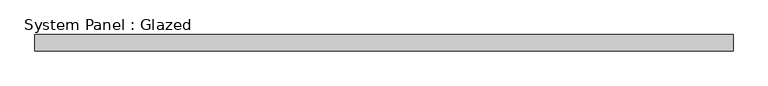
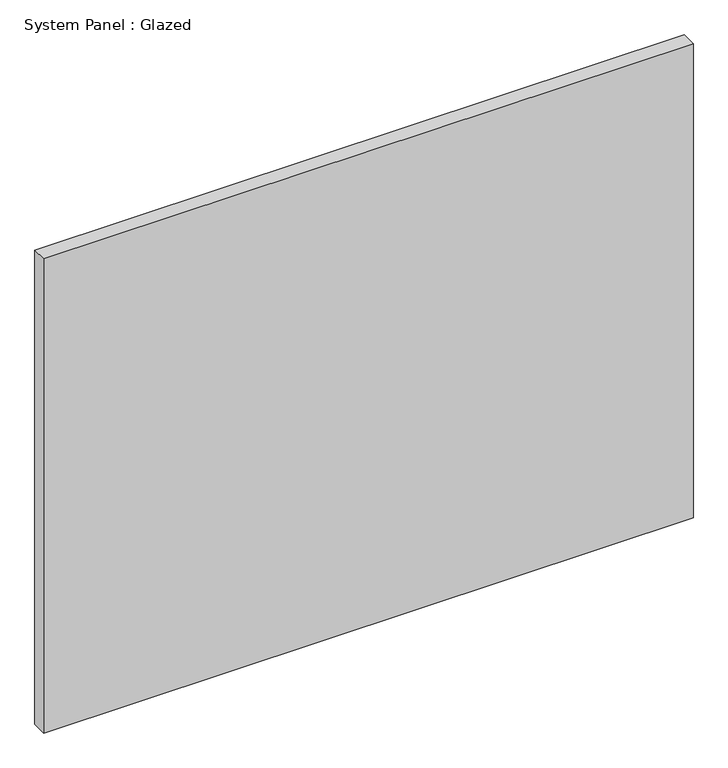
"""IFC4 building model written with IfcOpenShell, lengths in millimetres: plate geometry, System Panel : Glazed."""

from ifc_helpers import new_model, si_unit, origin, origin_with_axes, place, context, project, spatial, polyline, outline, extrude, source, transform, mapped, element, save


def system_panel_glazed_4667a6f9(model_context):
    return source(origin(), model_context, "Body", "SweptSolid", [
        extrude(outline(polyline([(549.2750001, 19.05), (-549.2750001, 19.05), (-549.2750001, 44.45), (549.2750001, 44.45), (549.2750001, 19.05)])), origin_with_axes(), (0.0, 0.0, 1.0), 847.5210507),
    ])


if __name__ == "__main__":
    model = new_model("IFC4")
    model_context = context("Model", 3, world=origin())
    ifc_project = project(units=[si_unit("LENGTHUNIT", "METRE", prefix="MILLI")], contexts=[model_context])
    site = spatial("IfcSite", under=ifc_project)
    building = spatial("IfcBuilding", under=site)
    placement = place(None, origin())
    system_panel_glazed_shape = system_panel_glazed_4667a6f9(model_context)
    element("IfcPlate", 1, ObjectType="System Panel : Glazed", at=placement, inside=building, context=model_context, shape_type="MappedRepresentation", body=[
        mapped(system_panel_glazed_shape, transform((0.0, 0.0, 0.0), x_axis=(1.0, 0.0, 0.0), y_axis=(0.0, 1.0, 0.0), z_axis=(0.0, 0.0, 1.0))),
    ])
    save(model, "model.ifc")

# Revit data of these elements
# Type "System Panel : Glazed"
#   Construction Type Id = "GSP4R"
#   Analytic Construction = "1/8 in Pilkington single glazing"
#   Visual Light Transmittance = 0.9
#   Solar Heat Gain Coefficient = 0.86
#   Heat Transfer Coefficient (U) = 1.18115 BTU/(h·ft²·°F)
#   Define Thermal Properties by = 1
# Element 1 (IfcPlate, "System Panel : Glazed")
#   Materials on its faces: "Glass"
# Materials
#   "Glass": class "Glass", colour RGB 0 128 192, transparency 0.75, Description = "Soda Lime Glass", Cost = 0
